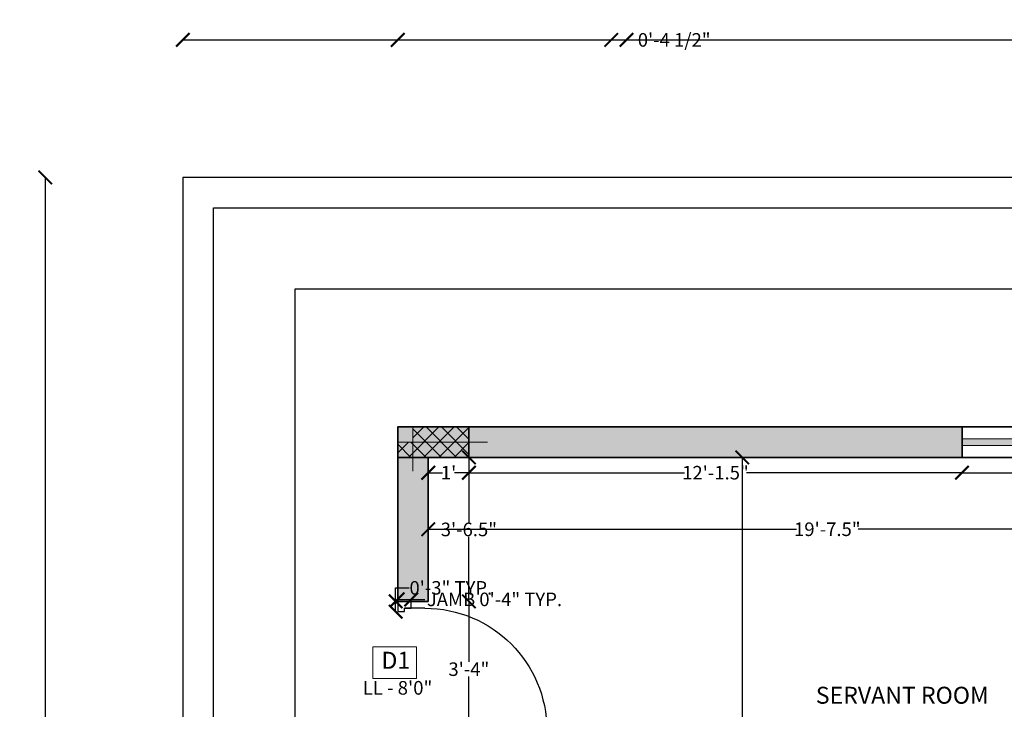
# Model space of a CAD drawing. Units: inches. Extents: x 2 to 905, y 9 to 678.
# Tile 5 of 8: x 5 to 295, y 474 to 678. Entities that reach past the tile are written whole.
import ezdxf

# ---------------------------------------------------------------- set-up
doc = ezdxf.new("R2010")
doc.units = ezdxf.units.IN
for name, color, linetype, lineweight in [('A-ANNO-DIMS', 7, 'Continuous', 18), ('A-COLS', 1, 'Continuous', 35), ('A-COLS-MARK', 1, 'Continuous', 18), ('A-COLS-PATT', 1, 'Continuous', 13), ('A-DOOR', 7, 'Continuous', 25), ('A-GLAZ', 4, 'Continuous', 18), ('A-WALL', 7, 'Continuous', 35), ('C-PROP', 7, 'Continuous', 25)]:
    doc.layers.add(name, color=color, linetype=linetype, lineweight=lineweight)
for name, color, linetype, lineweight, true_color in [('A-ANNO-IDEN', 251, 'Continuous', 18, 0x636466), ('A-AREA-IDEN', 252, 'Continuous', 18, 0x989898), ('A-WALL-PATT', 252, 'Continuous', 13, 0x939598)]:
    doc.layers.add(name, color=color, linetype=linetype, lineweight=lineweight, true_color=true_color)
doc.styles.add('PDF ArialMT', font='arial.ttf')
doc.styles.add('PDF Century Gothic Bold', font='txt')
doc.styles.get("Standard").update_dxf_attribs({"font": 'arial.ttf'})
doc.dimstyles.get("Standard").update_dxf_attribs({"dimtxt": 4, "dimasz": 4, "dimexe": 0.18, "dimexo": 0.0625, "dimgap": 0.09, "dimtad": 0, "dimtih": 1, "dimtoh": 1, "dimdec": 1, "dimzin": 0, "dimdsep": 46, "dimlunit": 3, "dimtxsty": 'Standard', "dimblk": 'ARCHTICK', "dimcen": 0, "dimse1": 1, "dimse2": 1, "dimclrt": 1, "dimadec": 0, "dimazin": 0, "dimtfac": 1, "dimtdec": 1, "dimtofl": 0, "dimtmove": 0, "dimatfit": 3, "dimfxl": 1, "dimtolj": 1, "dimtzin": 0, "dimarcsym": 0})

# ---------------------------------------------------------------- blocks, each defined once
blk = doc.blocks.new('*U5')
for p, q in [((0, 0), (0, -6)), ((36, 0), (36, -6))]:
    blk.add_line(p, q)
blk.add_lwpolyline([(0, 0), (0, 36), (1.75, 36), (1.75, 0)], close=True)
blk.add_arc((0, 0), 36, 0, 90)
blk = doc.blocks.new('_ArchTick')
at = {"color": 0, "linetype": 'ByBlock', "const_width": 0.15}
blk.add_lwpolyline([(-0.5, -0.5), (0.5, 0.5)], dxfattribs=at)
blk = doc.blocks.new('*D11')
at = {"layer": 'A-ANNO-DIMS', "color": 0, "lineweight": -2, "transparency": 16777216}
for p, q in [((218.07, 548.58), (218.07, 462.21)), ((218.07, 371.58), (218.07, 457.95))]:
    blk.add_line(p, q, dxfattribs=at)
at = {"layer": 'Defpoints', "color": 0, "transparency": 16777216}
for p in [(360.93, 548.58), (218.07, 371.58), (360.93, 371.58)]:
    blk.add_point(p, dxfattribs=at)
at = {"layer": 'A-ANNO-DIMS', "color": 0, "lineweight": -2, "transparency": 16777216, "xscale": 4, "yscale": 4, "zscale": 4}
for p, rotation in [((218.07, 548.58), 90), ((218.07, 371.58), 270)]:
    blk.add_blockref('_ArchTick', p, dxfattribs=dict(at, rotation=rotation))
at = {"layer": 'A-ANNO-DIMS', "color": 0, "transparency": 16777216, "insert": (218.07, 460.08), "char_height": 4, "attachment_point": 5}
blk.add_mtext('\\A1;14\'-9"', dxfattribs=at)
blk = doc.blocks.new('*D12')
at = {"layer": 'A-ANNO-DIMS', "color": 0, "lineweight": -2, "transparency": 16777216}
for p, q in [((125.43, 527.38), (234.08, 527.38)), ((360.93, 527.38), (252.29, 527.38))]:
    blk.add_line(p, q, dxfattribs=at)
at = {"layer": 'Defpoints', "color": 0, "transparency": 16777216}
for p in [(125.43, 548.58), (360.93, 548.58), (360.93, 527.38)]:
    blk.add_point(p, dxfattribs=at)
at = {"layer": 'A-ANNO-DIMS', "color": 0, "lineweight": -2, "transparency": 16777216, "xscale": 4, "yscale": 4, "zscale": 4, "rotation": 180}
blk.add_blockref('_ArchTick', (125.43, 527.38), dxfattribs=at)
at = {"layer": 'A-ANNO-DIMS', "color": 0, "lineweight": -2, "transparency": 16777216, "xscale": 4, "yscale": 4, "zscale": 4}
blk.add_blockref('_ArchTick', (360.93, 527.38), dxfattribs=at)
at = {"layer": 'A-ANNO-DIMS', "color": 0, "transparency": 16777216, "insert": (243.18, 527.38), "char_height": 4, "attachment_point": 5}
blk.add_mtext('\\A1;19\'-7.5"', dxfattribs=at)
blk = doc.blocks.new('*D54')
at = {"layer": 'A-ANNO-DIMS', "color": 0, "lineweight": -2, "transparency": 16777216}
for p, q in [((137.43, 506.08), (137.43, 488.21)), ((137.43, 466.08), (137.43, 483.94))]:
    blk.add_line(p, q, dxfattribs=at)
at = {"layer": 'Defpoints', "color": 0, "transparency": 16777216}
for p in [(132.75, 506.08), (137.43, 506.08), (132.75, 466.08)]:
    blk.add_point(p, dxfattribs=at)
at = {"layer": 'A-ANNO-DIMS', "color": 0, "lineweight": -2, "transparency": 16777216, "xscale": 4, "yscale": 4, "zscale": 4}
for p, rotation in [((137.43, 506.08), 90), ((137.43, 466.08), 270)]:
    blk.add_blockref('_ArchTick', p, dxfattribs=dict(at, rotation=rotation))
at = {"layer": 'A-ANNO-DIMS', "color": 0, "transparency": 16777216, "insert": (137.43, 486.08), "char_height": 4, "attachment_point": 5}
blk.add_mtext('\\A1;3\'-4"', dxfattribs=at)
blk = doc.blocks.new('*D55')
at = {"layer": 'A-ANNO-DIMS', "color": 0, "lineweight": -2, "transparency": 16777216}
for p, q in [((137.43, 548.58), (137.43, 529.46)), ((137.43, 506.08), (137.43, 525.19))]:
    blk.add_line(p, q, dxfattribs=at)
at = {"layer": 'Defpoints', "color": 0, "transparency": 16777216}
for p in [(132.75, 548.58), (137.43, 548.58), (132.75, 506.08)]:
    blk.add_point(p, dxfattribs=at)
at = {"layer": 'A-ANNO-DIMS', "color": 0, "lineweight": -2, "transparency": 16777216, "xscale": 4, "yscale": 4, "zscale": 4}
for p, rotation in [((137.43, 548.58), 90), ((137.43, 506.08), 270)]:
    blk.add_blockref('_ArchTick', p, dxfattribs=dict(at, rotation=rotation))
at = {"layer": 'A-ANNO-DIMS', "color": 0, "transparency": 16777216, "insert": (137.43, 527.33), "char_height": 4, "attachment_point": 5}
blk.add_mtext('\\A1;3\'-6.5"', dxfattribs=at)
blk = doc.blocks.new('*D56')
at = {"layer": 'A-ANNO-DIMS', "color": 0, "lineweight": -2, "transparency": 16777216}
for p, q in [((125.43, 544.07), (129.69, 544.07)), ((137.43, 544.07), (133.18, 544.07))]:
    blk.add_line(p, q, dxfattribs=at)
at = {"layer": 'Defpoints', "color": 0, "transparency": 16777216}
for p in [(125.43, 548.58), (137.43, 548.58), (137.43, 544.07)]:
    blk.add_point(p, dxfattribs=at)
at = {"layer": 'A-ANNO-DIMS', "color": 0, "lineweight": -2, "transparency": 16777216, "xscale": 4, "yscale": 4, "zscale": 4, "rotation": 180}
blk.add_blockref('_ArchTick', (125.43, 544.07), dxfattribs=at)
at = {"layer": 'A-ANNO-DIMS', "color": 0, "lineweight": -2, "transparency": 16777216, "xscale": 4, "yscale": 4, "zscale": 4}
blk.add_blockref('_ArchTick', (137.43, 544.07), dxfattribs=at)
at = {"layer": 'A-ANNO-DIMS', "color": 0, "transparency": 16777216, "insert": (131.43, 544.07), "char_height": 4, "attachment_point": 5}
blk.add_mtext("\\A1;1'", dxfattribs=at)
blk = doc.blocks.new('*D57')
at = {"layer": 'A-ANNO-DIMS', "color": 0, "lineweight": -2, "transparency": 16777216}
for p, q in [((137.43, 544.07), (201.08, 544.07)), ((282.93, 544.07), (219.29, 544.07))]:
    blk.add_line(p, q, dxfattribs=at)
at = {"layer": 'Defpoints', "color": 0, "transparency": 16777216}
for p in [(137.43, 548.58), (282.93, 548.58), (282.93, 544.07)]:
    blk.add_point(p, dxfattribs=at)
at = {"layer": 'A-ANNO-DIMS', "color": 0, "lineweight": -2, "transparency": 16777216, "xscale": 4, "yscale": 4, "zscale": 4, "rotation": 180}
blk.add_blockref('_ArchTick', (137.43, 544.07), dxfattribs=at)
at = {"layer": 'A-ANNO-DIMS', "color": 0, "lineweight": -2, "transparency": 16777216, "xscale": 4, "yscale": 4, "zscale": 4}
blk.add_blockref('_ArchTick', (282.93, 544.07), dxfattribs=at)
at = {"layer": 'A-ANNO-DIMS', "color": 0, "transparency": 16777216, "insert": (210.18, 544.07), "char_height": 4, "attachment_point": 5}
blk.add_mtext('\\A1;12\'-1.5"', dxfattribs=at)
blk = doc.blocks.new('*D58')
at = {"layer": 'A-ANNO-DIMS', "color": 0, "lineweight": -2, "transparency": 16777216}
for p, q in [((282.93, 544.07), (304.92, 544.07)), ((330.93, 544.07), (308.94, 544.07))]:
    blk.add_line(p, q, dxfattribs=at)
at = {"layer": 'Defpoints', "color": 0, "transparency": 16777216}
for p in [(282.93, 548.58), (330.93, 548.58), (330.93, 544.07)]:
    blk.add_point(p, dxfattribs=at)
at = {"layer": 'A-ANNO-DIMS', "color": 0, "lineweight": -2, "transparency": 16777216, "xscale": 4, "yscale": 4, "zscale": 4, "rotation": 180}
blk.add_blockref('_ArchTick', (282.93, 544.07), dxfattribs=at)
at = {"layer": 'A-ANNO-DIMS', "color": 0, "lineweight": -2, "transparency": 16777216, "xscale": 4, "yscale": 4, "zscale": 4}
blk.add_blockref('_ArchTick', (330.93, 544.07), dxfattribs=at)
at = {"layer": 'A-ANNO-DIMS', "color": 0, "transparency": 16777216, "insert": (306.93, 544.07), "char_height": 4, "attachment_point": 5}
blk.add_mtext("\\A1;4'", dxfattribs=at)
blk = doc.blocks.new('COL-DATUM-L')
h = blk.add_hatch(color=256)
h.dxf.hatch_style = 1
h.paths.add_polyline_path([(4.5, 0), (4.5, 4.5), (0, 4.5), (0, 0)])
for p, q in [((4.5, 0), (4.5, 26.48)), ((0, 4.5), (13.01, 4.5))]:
    blk.add_line(p, q)
blk.add_lwpolyline([(4.5, 0), (0, 0), (0, 4.5), (4.5, 4.5)], close=True)
blk = doc.blocks.new('GLAZ-W4-48')
h = blk.add_hatch(color=256)
h.dxf.hatch_style = 1
h.paths.add_polyline_path([(48, 0), (48, 2), (0, 2), (0, 0)])
for p, q in [((0, 2), (48, 2)), ((0, 0), (48, 0))]:
    blk.add_line(p, q)
blk = doc.blocks.new('DOOR-JAMB-REBATED')
blk.add_lwpolyline([(0, 0), (2, 0), (2, 1), (4, 1), (4, 3), (0, 3)], close=True)
blk = doc.blocks.new('*D100')
at = {"layer": 'A-ANNO-DIMS', "color": 0, "lineweight": -2, "transparency": 16777216}
for p, q in [((116.43, 506.68), (120.43, 506.68)), ((120.43, 506.68), (124.43, 506.68))]:
    blk.add_line(p, q, dxfattribs=at)
at = {"layer": 'Defpoints', "color": 0, "transparency": 16777216}
for p in [(116.43, 506.08), (120.43, 506.68), (120.43, 506.08)]:
    blk.add_point(p, dxfattribs=at)
at = {"layer": 'A-ANNO-DIMS', "color": 0, "lineweight": -2, "transparency": 16777216, "xscale": 4, "yscale": 4, "zscale": 4, "rotation": 180}
blk.add_blockref('_ArchTick', (116.43, 506.68), dxfattribs=at)
at = {"layer": 'A-ANNO-DIMS', "color": 0, "lineweight": -2, "transparency": 16777216, "xscale": 4, "yscale": 4, "zscale": 4}
blk.add_blockref('_ArchTick', (120.43, 506.68), dxfattribs=at)
at = {"layer": 'A-ANNO-DIMS', "color": 1, "transparency": 16777216, "insert": (144.98, 506.68), "char_height": 4, "attachment_point": 5}
blk.add_mtext('\\A1;JAMB 0\'-4" TYP.', dxfattribs=at)
blk = doc.blocks.new('*D101')
at = {"layer": 'A-ANNO-DIMS', "color": 0, "lineweight": -2, "transparency": 16777216}
for p, q in [((115.83, 506.08), (115.83, 510.08)), ((115.83, 510.08), (119.83, 510.08)), ((115.83, 503.08), (115.83, 506.08))]:
    blk.add_line(p, q, dxfattribs=at)
at = {"layer": 'Defpoints', "color": 0, "transparency": 16777216}
for p in [(115.83, 506.08), (116.43, 506.08), (116.43, 503.08)]:
    blk.add_point(p, dxfattribs=at)
at = {"layer": 'A-ANNO-DIMS', "color": 0, "lineweight": -2, "transparency": 16777216, "xscale": 4, "yscale": 4, "zscale": 4}
for p, rotation in [((115.83, 506.08), 90), ((115.83, 503.08), 270)]:
    blk.add_blockref('_ArchTick', p, dxfattribs=dict(at, rotation=rotation))
at = {"layer": 'A-ANNO-DIMS', "color": 1, "transparency": 16777216, "insert": (132.11, 510.08), "char_height": 4, "attachment_point": 5}
blk.add_mtext('\\A1;0\'-3" TYP.', dxfattribs=at)
blk = doc.blocks.new('*D102')
at = {"layer": 'A-ANNO-DIMS', "color": 0, "lineweight": -2, "transparency": 16777216}
for p, q in [((53.05, 671.82), (448.08, 671.82)), ((857.05, 671.82), (462.03, 671.82))]:
    blk.add_line(p, q, dxfattribs=at)
at = {"layer": 'Defpoints', "color": 0, "transparency": 16777216}
for p in [(857.05, 671.82), (53.05, 631.22), (857.05, 631.22)]:
    blk.add_point(p, dxfattribs=at)
at = {"layer": 'A-ANNO-DIMS', "color": 0, "lineweight": -2, "transparency": 16777216, "xscale": 4, "yscale": 4, "zscale": 4, "rotation": 180}
blk.add_blockref('_ArchTick', (53.05, 671.82), dxfattribs=at)
at = {"layer": 'A-ANNO-DIMS', "color": 0, "lineweight": -2, "transparency": 16777216, "xscale": 4, "yscale": 4, "zscale": 4}
blk.add_blockref('_ArchTick', (857.05, 671.82), dxfattribs=at)
at = {"layer": 'A-ANNO-DIMS', "color": 1, "transparency": 16777216, "insert": (455.05, 671.82), "char_height": 4, "attachment_point": 5}
blk.add_mtext('\\A1;67\'-0"', dxfattribs=at)
blk = doc.blocks.new('*D103')
at = {"layer": 'A-ANNO-DIMS', "color": 0, "lineweight": -2, "transparency": 16777216}
for p, q in [((12.45, 631.22), (12.45, 345.35)), ((12.45, 55.22), (12.45, 341.09))]:
    blk.add_line(p, q, dxfattribs=at)
at = {"layer": 'Defpoints', "color": 0, "transparency": 16777216}
for p in [(12.45, 631.22), (53.05, 631.22), (53.05, 55.22)]:
    blk.add_point(p, dxfattribs=at)
at = {"layer": 'A-ANNO-DIMS', "color": 0, "lineweight": -2, "transparency": 16777216, "xscale": 4, "yscale": 4, "zscale": 4}
for p, rotation in [((12.45, 631.22), 90), ((12.45, 55.22), 270)]:
    blk.add_blockref('_ArchTick', p, dxfattribs=dict(at, rotation=rotation))
at = {"layer": 'A-ANNO-DIMS', "color": 1, "transparency": 16777216, "insert": (12.45, 343.22), "char_height": 4, "attachment_point": 5}
blk.add_mtext('\\A1;48\'-0"', dxfattribs=at)
blk = doc.blocks.new('*D107')
at = {"layer": 'A-ANNO-DIMS', "color": 0, "lineweight": -2, "transparency": 16777216}
for p, q in [((62.05, 14.62), (68.61, 14.62)), ((86.05, 14.62), (79.49, 14.62))]:
    blk.add_line(p, q, dxfattribs=at)
at = {"layer": 'Defpoints', "color": 0, "transparency": 16777216}
for p in [(62.05, 622.22), (86.05, 598.22), (86.05, 14.62)]:
    blk.add_point(p, dxfattribs=at)
at = {"layer": 'A-ANNO-DIMS', "color": 0, "lineweight": -2, "transparency": 16777216, "xscale": 4, "yscale": 4, "zscale": 4, "rotation": 180}
blk.add_blockref('_ArchTick', (62.05, 14.62), dxfattribs=at)
at = {"layer": 'A-ANNO-DIMS', "color": 0, "lineweight": -2, "transparency": 16777216, "xscale": 4, "yscale": 4, "zscale": 4}
blk.add_blockref('_ArchTick', (86.05, 14.62), dxfattribs=at)
at = {"layer": 'A-ANNO-DIMS', "color": 1, "transparency": 16777216, "insert": (74.05, 14.62), "char_height": 4, "attachment_point": 5}
blk.add_mtext('\\A1;2\'-0"', dxfattribs=at)
blk = doc.blocks.new('*D108')
at = {"layer": 'A-ANNO-DIMS', "color": 0, "lineweight": -2, "transparency": 16777216}
for p, q in [((897.65, 622.22), (897.65, 612.35)), ((897.65, 598.22), (897.65, 608.09))]:
    blk.add_line(p, q, dxfattribs=at)
at = {"layer": 'Defpoints', "color": 0, "transparency": 16777216}
for p in [(62.05, 622.22), (86.05, 598.22), (897.65, 598.22)]:
    blk.add_point(p, dxfattribs=at)
at = {"layer": 'A-ANNO-DIMS', "color": 0, "lineweight": -2, "transparency": 16777216, "xscale": 4, "yscale": 4, "zscale": 4}
for p, rotation in [((897.65, 622.22), 90), ((897.65, 598.22), 270)]:
    blk.add_blockref('_ArchTick', p, dxfattribs=dict(at, rotation=rotation))
at = {"layer": 'A-ANNO-DIMS', "color": 1, "transparency": 16777216, "insert": (897.65, 610.22), "char_height": 4, "attachment_point": 5}
blk.add_mtext('\\A1;2\'-0"', dxfattribs=at)
blk = doc.blocks.new('*D111')
at = {"layer": 'A-ANNO-DIMS', "color": 0, "lineweight": -2, "transparency": 16777216}
for p, q in [((116.43, 671.82), (429.56, 671.82)), ((765.93, 671.82), (452.8, 671.82))]:
    blk.add_line(p, q, dxfattribs=at)
at = {"layer": 'Defpoints', "color": 0, "transparency": 16777216}
for p in [(765.93, 671.82), (116.43, 557.58), (765.93, 557.58)]:
    blk.add_point(p, dxfattribs=at)
at = {"layer": 'A-ANNO-DIMS', "color": 0, "lineweight": -2, "transparency": 16777216, "xscale": 4, "yscale": 4, "zscale": 4, "rotation": 180}
blk.add_blockref('_ArchTick', (116.43, 671.82), dxfattribs=at)
at = {"layer": 'A-ANNO-DIMS', "color": 0, "lineweight": -2, "transparency": 16777216, "xscale": 4, "yscale": 4, "zscale": 4}
blk.add_blockref('_ArchTick', (765.93, 671.82), dxfattribs=at)
at = {"layer": 'A-ANNO-DIMS', "color": 1, "transparency": 16777216, "insert": (441.18, 671.82), "char_height": 4, "attachment_point": 5}
blk.add_mtext('\\A1;54\'-1 1/2"', dxfattribs=at)
blk = doc.blocks.new('*D120')
at = {"layer": 'A-ANNO-DIMS', "color": 0, "lineweight": -2, "transparency": 16777216}
for p, q in [((179.43, 671.82), (183.93, 671.82)), ((183.93, 671.82), (187.93, 671.82))]:
    blk.add_line(p, q, dxfattribs=at)
at = {"layer": 'Defpoints', "color": 0, "transparency": 16777216}
for p in [(183.93, 671.82), (183.93, 460.08), (179.43, 455.58)]:
    blk.add_point(p, dxfattribs=at)
at = {"layer": 'A-ANNO-DIMS', "color": 0, "lineweight": -2, "transparency": 16777216, "xscale": 4, "yscale": 4, "zscale": 4, "rotation": 180}
blk.add_blockref('_ArchTick', (179.43, 671.82), dxfattribs=at)
at = {"layer": 'A-ANNO-DIMS', "color": 0, "lineweight": -2, "transparency": 16777216, "xscale": 4, "yscale": 4, "zscale": 4}
blk.add_blockref('_ArchTick', (183.93, 671.82), dxfattribs=at)
at = {"layer": 'A-ANNO-DIMS', "color": 1, "transparency": 16777216, "insert": (198, 671.82), "char_height": 4, "attachment_point": 5}
blk.add_mtext('\\A1;0\'-4 1/2"', dxfattribs=at)

msp = doc.modelspace()

# ---------------------------------------------------------------- hatches: boundary and pattern name
at = {"layer": 'A-COLS-PATT'}
h = msp.add_hatch(dxfattribs=at)
h.set_pattern_fill('ANSI37', color=256, angle=-90)
h.set_pattern_definition([(315, (-219.034, -221.098), (2.245064, 2.245064), []), (45, (-219.034, -221.098), (-2.245064, 2.245064), [])])
h.paths.add_polyline_path([(120.93, 548.58), (120.93, 553.08), (116.43, 553.08), (116.43, 548.58)])
h.paths.add_polyline_path([(137.43, 548.58), (137.43, 553.08), (120.93, 553.08), (120.93, 548.58)])
h.paths.add_polyline_path([(137.43, 553.08), (137.43, 557.58), (120.93, 557.58), (120.93, 553.08)])
at = {"layer": 'A-WALL-PATT'}
h = msp.add_hatch(color=256, dxfattribs=at)
h.dxf.hatch_style = 1
h.paths.add_polyline_path([(125.43, 227.58), (116.43, 227.58), (116.43, 128.58), (237.93, 128.58), (237.93, 137.58), (125.43, 137.58)])
h.paths.add_polyline_path([(249.93, 302.58), (183.93, 302.58), (183.93, 320.58), (179.43, 320.58), (179.43, 302.58), (116.43, 302.58), (116.43, 275.58), (125.43, 275.58), (125.43, 293.58), (249.93, 293.58), (249.93, 297.58)], flags=0)
h.paths.add_polyline_path([(369.93, 137.58), (360.93, 137.58), (360.93, 218.58), (369.93, 218.58), (369.93, 227.58), (363.93, 227.58), (351.93, 227.58), (351.93, 137.58), (345.93, 137.58), (345.93, 128.58), (360.93, 128.58), (369.93, 128.58)])
h.paths.add_polyline_path([(297.93, 137.58), (285.93, 137.58), (285.93, 128.58), (297.93, 128.58)])
h.paths.add_polyline_path([(369.93, 444.58), (360.93, 444.58), (360.93, 371.58), (183.93, 371.58), (183.93, 460.08), (125.43, 460.08), (125.43, 466.08), (116.43, 466.08), (116.43, 449.58), (120.43, 449.58), (125.43, 449.58), (125.43, 455.58), (179.43, 455.58), (179.43, 371.58), (125.43, 371.58), (125.43, 389.58), (116.43, 389.58), (116.43, 362.58), (179.43, 362.58), (179.43, 344.58), (183.93, 344.58), (183.93, 362.58), (291.93, 362.58), (291.93, 302.58), (285.93, 302.58), (285.93, 293.58), (309.93, 293.58), (309.93, 302.58), (300.93, 302.58), (300.93, 362.58), (360.93, 362.58), (360.93, 302.58), (351.93, 302.58), (351.93, 293.58), (360.93, 293.58), (360.93, 275.58), (363.93, 275.58), (369.93, 275.58)])
h.paths.add_polyline_path([(282.93, 557.58), (116.43, 557.58), (116.43, 506.08), (120.43, 506.08), (125.43, 506.08), (125.43, 548.58), (282.93, 548.58)])
h.paths.add_polyline_path([(369.93, 557.58), (330.93, 557.58), (330.93, 548.58), (360.93, 548.58), (360.93, 504.58), (369.93, 504.58)])

# ---------------------------------------------------------------- linework, layer by layer
at = {"layer": 'A-ANNO-IDEN'}
msp.add_lwpolyline([(109.07, 492.7), (121.97, 492.7), (121.97, 483.33), (109.07, 483.33)], close=True, dxfattribs=at)
at = {"layer": 'A-COLS'}
msp.add_lwpolyline([(137.43, 557.58), (137.43, 548.58), (116.43, 548.58), (116.43, 557.58)], close=True, dxfattribs=at)
at = {"layer": 'A-GLAZ'}
msp.add_lwpolyline([(282.93, 557.58), (330.93, 557.58), (330.93, 548.58), (282.93, 548.58)], close=True, dxfattribs=at)
at = {"layer": 'A-WALL'}
for p, q in [((282.93, 548.58), (282.93, 557.58)), ((282.93, 557.58), (282.93, 548.58))]:
    msp.add_line(p, q, dxfattribs=at)
msp.add_lwpolyline([(125.43, 506.08), (116.43, 506.08), (116.43, 557.58), (369.93, 557.58), (369.93, 504.58), (360.93, 504.58), (369.93, 504.58), (360.93, 504.58), (360.93, 548.58), (125.43, 548.58)], close=True, dxfattribs=at)
at = {"layer": 'C-PROP'}
msp.add_lwpolyline([(857.05, 535.22), (857.05, 631.22), (53.05, 631.22), (53.05, 55.22), (857.05, 55.22), (857.05, 355.22), (848.05, 355.22), (848.05, 64.22), (62.05, 64.22), (62.05, 622.22), (848.05, 622.22), (848.05, 535.22)], close=True, dxfattribs=at)
msp.add_lwpolyline([(848.05, 598.22), (86.05, 598.22), (86.05, 88.22), (824.05, 88.22), (824.05, 355.22), (836.05, 355.22), (848.05, 355.22)], dxfattribs=at)

# ---------------------------------------------------------------- block references
at = {"layer": 'A-COLS-MARK', "rotation": 269.9999999999998}
msp.add_blockref('COL-DATUM-L', (116.43, 557.58), dxfattribs=at)
at = {"layer": 'A-DOOR'}
msp.add_blockref('DOOR-JAMB-REBATED', (116.43, 503.08), dxfattribs=at)
at = {"layer": 'A-DOOR', "xscale": -1, "rotation": 270}
msp.add_blockref('*U5', (124.43, 468.08), dxfattribs=at)
at = {"layer": 'A-GLAZ'}
msp.add_blockref('GLAZ-W4-48', (282.93, 552.08), dxfattribs=at)

# ---------------------------------------------------------------- texts
at = {"layer": 'A-ANNO-IDEN', "attachment_point": 4, "style": 'PDF ArialMT'}
for s, insert, char_height in [('D1', (111.62, 488.05), 5.029), ('LL - 8\'0"', (106.11, 480.05), 4.023)]:
    msp.add_mtext(s, dxfattribs=dict(at, insert=insert, char_height=char_height))
at = {"layer": 'A-AREA-IDEN', "insert": (239.78, 477.74), "char_height": 5, "attachment_point": 4, "style": 'PDF Century Gothic Bold'}
msp.add_mtext('SERVANT ROOM', dxfattribs=at)

# ---------------------------------------------------------------- dimensions: what is measured, and where the dimension line sits
at = {"layer": 'A-ANNO-DIMS'}
for base, p1, p2, override, picture, middle in [((765.93, 671.82), (116.43, 557.58), (765.93, 557.58), {"dimdec": 1, "dimlfac": 1, "dimrnd": 0, "dimzin": 1, "dimdsep": 46, "dimlunit": 4, "dimfrac": 2}, '*D111', (441.18, 671.82)), ((183.93, 671.82), (179.43, 455.58), (183.93, 460.08), {"dimdec": 1, "dimlfac": 1, "dimrnd": 0, "dimzin": 1, "dimdsep": 46, "dimlunit": 4, "dimfrac": 2}, '*D120', (198, 671.82)), ((857.05, 671.82), (53.05, 631.22), (857.05, 631.22), {"dimdec": 1, "dimlfac": 1, "dimrnd": 0, "dimzin": 1, "dimdsep": 46, "dimlunit": 4, "dimfrac": 2}, '*D102', (455.05, 671.82)), ((86.05, 14.62), (62.05, 622.22), (86.05, 598.22), {"dimdec": 1, "dimlfac": 1, "dimrnd": 0, "dimzin": 1, "dimdsep": 46, "dimlunit": 4, "dimfrac": 2}, '*D107', (74.05, 14.62)), ((360.93, 527.38), (125.43, 548.58), (360.93, 548.58), {"dimclrd": 0, "dimclre": 0, "dimclrt": 0}, '*D12', (243.18, 527.38)), ((137.43, 544.07), (125.43, 548.58), (137.43, 548.58), {"dimclrd": 0, "dimclre": 0, "dimclrt": 0}, '*D56', (131.43, 544.07)), ((282.93, 544.07), (137.43, 548.58), (282.93, 548.58), {"dimclrd": 0, "dimclre": 0, "dimclrt": 0, "dimtmove": 1}, '*D57', (210.18, 544.07)), ((330.93, 544.07), (282.93, 548.58), (330.93, 548.58), {"dimclrd": 0, "dimclre": 0, "dimclrt": 0, "dimtmove": 1}, '*D58', (306.93, 544.07))]:
    dim = msp.add_linear_dim(base=base, p1=p1, p2=p2, dimstyle='Standard', override=override, dxfattribs=at)
    dim.commit()
    dim.dimension.update_dxf_attribs({"geometry": picture, "text_midpoint": middle})
for base, p1, p2, override, picture, middle in [((12.45, 631.22), (53.05, 55.22), (53.05, 631.22), {"dimdec": 1, "dimlfac": 1, "dimrnd": 0, "dimzin": 1, "dimdsep": 46, "dimlunit": 4, "dimfrac": 2}, '*D103', (12.45, 343.22)), ((897.65, 598.22), (62.05, 622.22), (86.05, 598.22), {"dimdec": 1, "dimlfac": 1, "dimrnd": 0, "dimzin": 1, "dimdsep": 46, "dimlunit": 4, "dimfrac": 2}, '*D108', (897.65, 610.22)), ((137.43, 548.58), (132.75, 506.08), (132.75, 548.58), {"dimclrd": 0, "dimclre": 0, "dimclrt": 0, "dimtmove": 1}, '*D55', (137.43, 527.33)), ((218.07, 371.58), (360.93, 548.58), (360.93, 371.58), {"dimdec": 0, "dimclrd": 0, "dimclre": 0, "dimclrt": 0}, '*D11', (218.07, 460.08)), ((137.43, 506.08), (132.75, 466.08), (132.75, 506.08), {"dimdec": 0, "dimclrd": 0, "dimclre": 0, "dimclrt": 0, "dimtmove": 1}, '*D54', (137.43, 486.08))]:
    dim = msp.add_linear_dim(base=base, p1=p1, p2=p2, angle=90, dimstyle='Standard', override=override, dxfattribs=at)
    dim.commit()
    dim.dimension.update_dxf_attribs({"geometry": picture, "text_midpoint": middle})
dim = msp.add_linear_dim(base=(115.83, 506.08), p1=(116.43, 503.08), p2=(116.43, 506.08), angle=90, text='<> TYP.', dimstyle='Standard', override={"dimdec": 1, "dimlfac": 1, "dimrnd": 0, "dimzin": 1, "dimdsep": 46, "dimlunit": 4, "dimfrac": 2}, dxfattribs=at)
dim.commit()
dim.dimension.update_dxf_attribs({"geometry": '*D101', "text_midpoint": (132.11, 510.08)})
dim = msp.add_linear_dim(base=(120.43, 506.68), p1=(116.43, 506.08), p2=(120.43, 506.08), text='JAMB <> TYP.', dimstyle='Standard', override={"dimdec": 1, "dimlfac": 1, "dimrnd": 0, "dimzin": 1, "dimdsep": 46, "dimlunit": 4, "dimfrac": 2}, dxfattribs=at)
dim.commit()
dim.dimension.update_dxf_attribs({"geometry": '*D100', "text_midpoint": (144.98, 506.68)})

doc.saveas('drawing.dxf')
